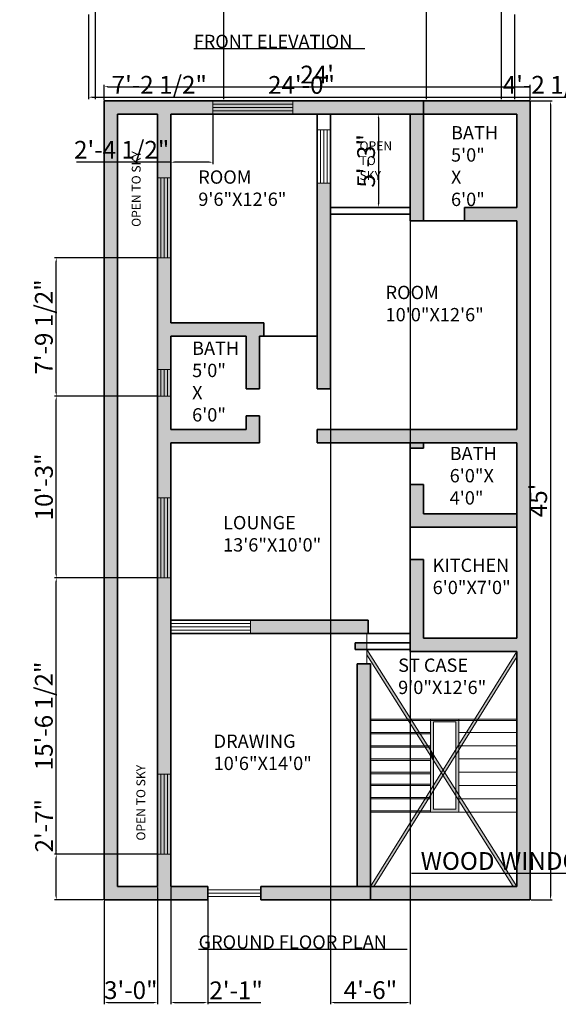
# Model space of a CAD drawing. Units: inches. Extents: x 2693 to 3501, y 1190 to 2292.
# Tile 1 of 4: x 2704 to 3068, y 1192 to 1858. Entities that reach past the tile are written whole.
import ezdxf

# ---------------------------------------------------------------- set-up
doc = ezdxf.new("R2010")
doc.units = ezdxf.units.IN
for name, color, linetype, lineweight in [('A-ANNO-DIMS', 2, 'Continuous', 18), ('A-ANNO-TEXT', 7, 'Continuous', 25), ('A-AREA-IDEN', 7, 'Continuous', 18), ('A-FLOR-STRS', 7, 'Continuous', 18), ('A-FLOR-STRS-PATT', 252, 'Continuous', 13), ('A-GLAZ', 4, 'Continuous', 18), ('A-WALL', 7, 'Continuous', 35), ('A-WALL-PATT', 252, 'Continuous', 13)]:
    doc.layers.add(name, color=color, linetype=linetype, lineweight=lineweight)
doc.styles.get("Standard").update_dxf_attribs({"font": 'arial.ttf'})
doc.dimstyles.new('ISO-25', dxfattribs={"dimtxt": 12, "dimasz": 2.5, "dimexe": 1.25, "dimexo": 0.625, "dimtad": 1, "dimdec": 1, "dimlunit": 3, "dimtxsty": 'Standard', "dimcen": 2.5, "dimadec": 0, "dimazin": 0, "dimtfac": 1, "dimtdec": 1, "dimtmove": 0, "dimatfit": 3, "dimfxl": 1, "dimarcsym": 0})

# ---------------------------------------------------------------- blocks, each defined once
blk = doc.blocks.new('Window - Wood Frame 36 in. Wide plan')
for p, q in [((0, 6), (0, 0)), ((0, 4.5), (36, 4.5)), ((36, 6), (36, 0)), ((0, 3), (36, 3)), ((0, 1.5), (36, 1.5))]:
    blk.add_line(p, q)
blk = doc.blocks.new('*D3')
at = {"layer": 'A-ANNO-DIMS', "color": 0, "lineweight": -2, "transparency": 16777216}
for p, q in [((2761.25, 1803.64), (2761.25, 1813.89)), ((2763.75, 1812.64), (3046.75, 1812.64)), ((3049.25, 1803.64), (3049.25, 1813.89))]:
    blk.add_line(p, q, dxfattribs=at)
at = {"layer": 'A-ANNO-DIMS', "color": 0, "transparency": 16777216}
for points in [[(2763.75, 1813.05), (2763.75, 1812.22), (2761.25, 1812.64)], [(3046.75, 1813.05), (3046.75, 1812.22), (3049.25, 1812.64)]]:
    blk.add_solid(points, dxfattribs=at)
at = {"layer": 'Defpoints', "color": 0, "transparency": 16777216}
for p in [(3049.25, 1812.64), (2761.25, 1803.02), (3049.25, 1803.02)]:
    blk.add_point(p, dxfattribs=at)
at = {"layer": 'A-ANNO-DIMS', "color": 0, "transparency": 16777216, "insert": (2905.25, 1819.29), "char_height": 12, "attachment_point": 5}
blk.add_mtext("24'", dxfattribs=at)
blk = doc.blocks.new('*D4')
at = {"layer": 'A-ANNO-DIMS', "color": 0, "lineweight": -2, "transparency": 16777216}
for p, q in [((3049.88, 1803.02), (3064.23, 1803.02)), ((3062.98, 1800.52), (3062.98, 1265.52)), ((3049.88, 1263.02), (3064.23, 1263.02))]:
    blk.add_line(p, q, dxfattribs=at)
at = {"layer": 'A-ANNO-DIMS', "color": 0, "transparency": 16777216}
for points in [[(3062.57, 1800.52), (3063.4, 1800.52), (3062.98, 1803.02)], [(3062.57, 1265.52), (3063.4, 1265.52), (3062.98, 1263.02)]]:
    blk.add_solid(points, dxfattribs=at)
at = {"layer": 'Defpoints', "color": 0, "transparency": 16777216}
for p in [(3049.25, 1803.02), (3049.25, 1263.02), (3062.98, 1263.02)]:
    blk.add_point(p, dxfattribs=at)
at = {"layer": 'A-ANNO-DIMS', "color": 0, "transparency": 16777216, "insert": (3056.26, 1533.02), "char_height": 12, "attachment_point": 5, "rotation": 90}
blk.add_mtext("45'", dxfattribs=at)
blk = doc.blocks.new('*D11')
at = {"layer": 'A-ANNO-DIMS', "color": 0, "lineweight": -2, "transparency": 16777216}
for p, q in [((3183.29, 1280.93), (2969.02, 1280.93)), ((3183.29, 1276.16), (3183.29, 1282.18)), ((3216.79, 1280.93), (3185.79, 1280.93)), ((3219.29, 1276.16), (3219.29, 1282.18))]:
    blk.add_line(p, q, dxfattribs=at)
at = {"layer": 'A-ANNO-DIMS', "color": 0, "transparency": 16777216}
for points in [[(3185.79, 1281.35), (3185.79, 1280.52), (3183.29, 1280.93)], [(3216.79, 1281.35), (3216.79, 1280.52), (3219.29, 1280.93)]]:
    blk.add_solid(points, dxfattribs=at)
at = {"layer": 'Defpoints', "color": 0, "transparency": 16777216}
for p in [(3183.29, 1280.93), (3183.29, 1275.53), (3219.29, 1275.53)]:
    blk.add_point(p, dxfattribs=at)
at = {"layer": 'A-ANNO-DIMS', "color": 0, "transparency": 16777216, "insert": (3074.91, 1287.77), "char_height": 12, "attachment_point": 5}
blk.add_mtext('WOOD WINDOW 3\'-0" TYP.', dxfattribs=at)
blk = doc.blocks.new('*D21')
at = {"layer": 'A-ANNO-DIMS', "color": 0, "lineweight": -2, "transparency": 16777216}
for p, q in [((2797.25, 1271.39), (2797.25, 1192.46)), ((2761.25, 1262.39), (2761.25, 1192.46)), ((2763.75, 1193.71), (2794.75, 1193.71))]:
    blk.add_line(p, q, dxfattribs=at)
at = {"layer": 'A-ANNO-DIMS', "color": 0, "transparency": 16777216}
for points in [[(2763.75, 1194.13), (2763.75, 1193.3), (2761.25, 1193.71)], [(2794.75, 1194.13), (2794.75, 1193.3), (2797.25, 1193.71)]]:
    blk.add_solid(points, dxfattribs=at)
at = {"layer": 'Defpoints', "color": 0, "transparency": 16777216}
for p in [(2797.25, 1272.02), (2761.25, 1263.02), (2797.25, 1193.71)]:
    blk.add_point(p, dxfattribs=at)
at = {"layer": 'A-ANNO-DIMS', "color": 0, "transparency": 16777216, "insert": (2779.25, 1200.47), "char_height": 12, "attachment_point": 5}
blk.add_mtext('3\'-0"', dxfattribs=at)
blk = doc.blocks.new('*D22')
at = {"layer": 'A-ANNO-DIMS', "color": 0, "lineweight": -2, "transparency": 16777216}
for p, q in [((2728.85, 1293.99), (2728.85, 1329.84)), ((2796.63, 1293.99), (2727.6, 1293.99)), ((2728.85, 1265.52), (2728.85, 1291.49)), ((2760.63, 1263.02), (2727.6, 1263.02))]:
    blk.add_line(p, q, dxfattribs=at)
at = {"layer": 'A-ANNO-DIMS', "color": 0, "transparency": 16777216}
for points in [[(2728.44, 1291.49), (2729.27, 1291.49), (2728.85, 1293.99)], [(2728.44, 1265.52), (2729.27, 1265.52), (2728.85, 1263.02)]]:
    blk.add_solid(points, dxfattribs=at)
at = {"layer": 'Defpoints', "color": 0, "transparency": 16777216}
for p in [(2728.85, 1293.99), (2797.25, 1293.99), (2761.25, 1263.02)]:
    blk.add_point(p, dxfattribs=at)
at = {"layer": 'A-ANNO-DIMS', "color": 0, "transparency": 16777216, "insert": (2722.2, 1313.17), "char_height": 12, "attachment_point": 5, "rotation": 90}
blk.add_mtext('2\'-7"', dxfattribs=at)
blk = doc.blocks.new('*D23')
at = {"layer": 'A-ANNO-DIMS', "color": 0, "lineweight": -2, "transparency": 16777216}
for p, q in [((2796.63, 1480.71), (2727.6, 1480.71)), ((2728.85, 1296.49), (2728.85, 1478.21)), ((2796.63, 1293.99), (2727.6, 1293.99))]:
    blk.add_line(p, q, dxfattribs=at)
at = {"layer": 'A-ANNO-DIMS', "color": 0, "transparency": 16777216}
for points in [[(2728.44, 1478.21), (2729.27, 1478.21), (2728.85, 1480.71)], [(2728.44, 1296.49), (2729.27, 1296.49), (2728.85, 1293.99)]]:
    blk.add_solid(points, dxfattribs=at)
at = {"layer": 'Defpoints', "color": 0, "transparency": 16777216}
for p in [(2728.85, 1480.71), (2797.25, 1480.71), (2797.25, 1293.99)]:
    blk.add_point(p, dxfattribs=at)
at = {"layer": 'A-ANNO-DIMS', "color": 0, "transparency": 16777216, "insert": (2722.02, 1387.35), "char_height": 12, "attachment_point": 5, "rotation": 90}
blk.add_mtext('15\'-6 1/2"', dxfattribs=at)
blk = doc.blocks.new('*D24')
at = {"layer": 'A-ANNO-DIMS', "color": 0, "lineweight": -2, "transparency": 16777216}
for p, q in [((2796.63, 1603.53), (2727.6, 1603.53)), ((2728.85, 1483.21), (2728.85, 1601.03)), ((2796.63, 1480.71), (2727.6, 1480.71))]:
    blk.add_line(p, q, dxfattribs=at)
at = {"layer": 'A-ANNO-DIMS', "color": 0, "transparency": 16777216}
for points in [[(2728.44, 1601.03), (2729.27, 1601.03), (2728.85, 1603.53)], [(2728.44, 1483.21), (2729.27, 1483.21), (2728.85, 1480.71)]]:
    blk.add_solid(points, dxfattribs=at)
at = {"layer": 'Defpoints', "color": 0, "transparency": 16777216}
for p in [(2728.85, 1603.53), (2797.25, 1603.53), (2797.25, 1480.71)]:
    blk.add_point(p, dxfattribs=at)
at = {"layer": 'A-ANNO-DIMS', "color": 0, "transparency": 16777216, "insert": (2722.1, 1542.12), "char_height": 12, "attachment_point": 5, "rotation": 90}
blk.add_mtext('10\'-3"', dxfattribs=at)
blk = doc.blocks.new('*D25')
at = {"layer": 'A-ANNO-DIMS', "color": 0, "lineweight": -2, "transparency": 16777216}
for p, q in [((2796.63, 1696.98), (2727.6, 1696.98)), ((2728.85, 1606.03), (2728.85, 1694.48)), ((2796.63, 1603.53), (2727.6, 1603.53))]:
    blk.add_line(p, q, dxfattribs=at)
at = {"layer": 'A-ANNO-DIMS', "color": 0, "transparency": 16777216}
for points in [[(2728.44, 1694.48), (2729.27, 1694.48), (2728.85, 1696.98)], [(2728.44, 1606.03), (2729.27, 1606.03), (2728.85, 1603.53)]]:
    blk.add_solid(points, dxfattribs=at)
at = {"layer": 'Defpoints', "color": 0, "transparency": 16777216}
for p in [(2728.85, 1696.98), (2797.25, 1696.98), (2797.25, 1603.53)]:
    blk.add_point(p, dxfattribs=at)
at = {"layer": 'A-ANNO-DIMS', "color": 0, "transparency": 16777216, "insert": (2722.02, 1650.25), "char_height": 12, "attachment_point": 5, "rotation": 90}
blk.add_mtext('7\'-9 1/2"', dxfattribs=at)
blk = doc.blocks.new('*D26')
at = {"layer": 'A-ANNO-DIMS', "color": 0, "lineweight": -2, "transparency": 16777216}
for p, q in [((2806.25, 1271.39), (2806.25, 1192.46)), ((2831.27, 1271.39), (2831.27, 1192.46)), ((2808.75, 1193.71), (2828.77, 1193.71)), ((2831.27, 1193.71), (2867.12, 1193.71))]:
    blk.add_line(p, q, dxfattribs=at)
at = {"layer": 'A-ANNO-DIMS', "color": 0, "transparency": 16777216}
for points in [[(2808.75, 1194.13), (2808.75, 1193.3), (2806.25, 1193.71)], [(2828.77, 1194.13), (2828.77, 1193.3), (2831.27, 1193.71)]]:
    blk.add_solid(points, dxfattribs=at)
at = {"layer": 'Defpoints', "color": 0, "transparency": 16777216}
for p in [(2806.25, 1272.02), (2831.27, 1272.02), (2831.27, 1193.71)]:
    blk.add_point(p, dxfattribs=at)
at = {"layer": 'A-ANNO-DIMS', "color": 0, "transparency": 16777216, "insert": (2850.45, 1200.36), "char_height": 12, "attachment_point": 5}
blk.add_mtext('2\'-1"', dxfattribs=at)
blk = doc.blocks.new('*D27')
at = {"layer": 'A-ANNO-DIMS', "color": 0, "lineweight": -2, "transparency": 16777216}
for p, q in [((2806.25, 1793.39), (2806.25, 1760.37)), ((2834.73, 1793.39), (2834.73, 1760.37)), ((2806.25, 1761.62), (2742.44, 1761.62)), ((2832.23, 1761.62), (2808.75, 1761.62))]:
    blk.add_line(p, q, dxfattribs=at)
at = {"layer": 'A-ANNO-DIMS', "color": 0, "transparency": 16777216}
for points in [[(2808.75, 1762.03), (2808.75, 1761.2), (2806.25, 1761.62)], [(2832.23, 1762.03), (2832.23, 1761.2), (2834.73, 1761.62)]]:
    blk.add_solid(points, dxfattribs=at)
at = {"layer": 'Defpoints', "color": 0, "transparency": 16777216}
for p in [(2806.25, 1794.02), (2834.73, 1794.02), (2806.25, 1761.62)]:
    blk.add_point(p, dxfattribs=at)
at = {"layer": 'A-ANNO-DIMS', "color": 0, "transparency": 16777216, "insert": (2773.1, 1768.45), "char_height": 12, "attachment_point": 5}
blk.add_mtext('2\'-4 1/2"', dxfattribs=at)
blk = doc.blocks.new('*D28')
at = {"layer": 'A-ANNO-DIMS', "color": 0, "lineweight": -2, "transparency": 16777216}
for p, q in [((2914.25, 1730.39), (2914.25, 1192.46)), ((2968.25, 1730.39), (2968.25, 1192.46)), ((2916.75, 1193.71), (2965.75, 1193.71))]:
    blk.add_line(p, q, dxfattribs=at)
at = {"layer": 'A-ANNO-DIMS', "color": 0, "transparency": 16777216}
for points in [[(2916.75, 1194.13), (2916.75, 1193.3), (2914.25, 1193.71)], [(2965.75, 1194.13), (2965.75, 1193.3), (2968.25, 1193.71)]]:
    blk.add_solid(points, dxfattribs=at)
at = {"layer": 'Defpoints', "color": 0, "transparency": 16777216}
for p in [(2914.25, 1731.02), (2968.25, 1731.02), (2968.25, 1193.71)]:
    blk.add_point(p, dxfattribs=at)
at = {"layer": 'A-ANNO-DIMS', "color": 0, "transparency": 16777216, "insert": (2941.25, 1200.47), "char_height": 12, "attachment_point": 5}
blk.add_mtext('4\'-6"', dxfattribs=at)
blk = doc.blocks.new('*D29')
at = {"layer": 'A-ANNO-DIMS', "color": 0, "lineweight": -2, "transparency": 16777216}
for p, q in [((2914.88, 1794.02), (2947.9, 1794.02)), ((2946.65, 1791.52), (2946.65, 1733.52)), ((2914.88, 1731.02), (2947.9, 1731.02))]:
    blk.add_line(p, q, dxfattribs=at)
at = {"layer": 'A-ANNO-DIMS', "color": 0, "transparency": 16777216}
for points in [[(2946.24, 1791.52), (2947.07, 1791.52), (2946.65, 1794.02)], [(2946.24, 1733.52), (2947.07, 1733.52), (2946.65, 1731.02)]]:
    blk.add_solid(points, dxfattribs=at)
at = {"layer": 'Defpoints', "color": 0, "transparency": 16777216}
for p in [(2914.25, 1794.02), (2914.25, 1731.02), (2946.65, 1731.02)]:
    blk.add_point(p, dxfattribs=at)
at = {"layer": 'A-ANNO-DIMS', "color": 0, "transparency": 16777216, "insert": (2939.9, 1762.52), "char_height": 12, "attachment_point": 5, "rotation": 90}
blk.add_mtext('5\'-3"', dxfattribs=at)
blk = doc.blocks.new('*D36')
at = {"layer": 'A-ANNO-DIMS', "color": 0, "lineweight": -2, "transparency": 16777216}
for p, q in [((2841.85, 1945.66), (2841.85, 1804.29)), ((2755.18, 1889.87), (2755.18, 1804.29)), ((2757.68, 1805.54), (2839.35, 1805.54))]:
    blk.add_line(p, q, dxfattribs=at)
at = {"layer": 'A-ANNO-DIMS', "color": 0, "transparency": 16777216}
for points in [[(2757.68, 1805.95), (2757.68, 1805.12), (2755.18, 1805.54)], [(2839.35, 1805.95), (2839.35, 1805.12), (2841.85, 1805.54)]]:
    blk.add_solid(points, dxfattribs=at)
at = {"layer": 'Defpoints', "color": 0, "transparency": 16777216}
for p in [(2841.85, 1946.28), (2755.18, 1890.49), (2841.85, 1805.54)]:
    blk.add_point(p, dxfattribs=at)
at = {"layer": 'A-ANNO-DIMS', "color": 0, "transparency": 16777216, "insert": (2798.51, 1812.37), "char_height": 12, "attachment_point": 5}
blk.add_mtext('7\'-2 1/2"', dxfattribs=at)
blk = doc.blocks.new('*D41')
at = {"layer": 'A-ANNO-DIMS', "color": 0, "lineweight": -2, "transparency": 16777216}
for p, q in [((2978.99, 1889.87), (2978.99, 1804.29)), ((3029.68, 1889.87), (3029.68, 1804.29)), ((2981.49, 1805.54), (3027.18, 1805.54)), ((3029.68, 1805.54), (3093.77, 1805.54))]:
    blk.add_line(p, q, dxfattribs=at)
at = {"layer": 'A-ANNO-DIMS', "color": 0, "transparency": 16777216}
for points in [[(2981.49, 1805.95), (2981.49, 1805.12), (2978.99, 1805.54)], [(3027.18, 1805.95), (3027.18, 1805.12), (3029.68, 1805.54)]]:
    blk.add_solid(points, dxfattribs=at)
at = {"layer": 'Defpoints', "color": 0, "transparency": 16777216}
for p in [(2978.99, 1890.49), (3029.68, 1890.49), (3029.68, 1805.54)]:
    blk.add_point(p, dxfattribs=at)
at = {"layer": 'A-ANNO-DIMS', "color": 0, "transparency": 16777216, "insert": (3062.97, 1812.37), "char_height": 12, "attachment_point": 5}
blk.add_mtext('4\'-2 1/2"', dxfattribs=at)
blk = doc.blocks.new('*D46')
at = {"layer": 'A-ANNO-DIMS', "color": 0, "lineweight": -2, "transparency": 16777216}
for p, q in [((2750.68, 1861.37), (2750.68, 1804.29)), ((3038.68, 1861.37), (3038.68, 1804.29)), ((2753.18, 1805.54), (3036.18, 1805.54))]:
    blk.add_line(p, q, dxfattribs=at)
at = {"layer": 'A-ANNO-DIMS', "color": 0, "transparency": 16777216}
for points in [[(2753.18, 1805.95), (2753.18, 1805.12), (2750.68, 1805.54)], [(3036.18, 1805.95), (3036.18, 1805.12), (3038.68, 1805.54)]]:
    blk.add_solid(points, dxfattribs=at)
at = {"layer": 'Defpoints', "color": 0, "transparency": 16777216}
for p in [(2750.68, 1861.99), (3038.68, 1861.99), (3038.68, 1805.54)]:
    blk.add_point(p, dxfattribs=at)
at = {"layer": 'A-ANNO-DIMS', "color": 0, "transparency": 16777216, "insert": (2894.68, 1812.29), "char_height": 12, "attachment_point": 5}
blk.add_mtext('24\'-0"', dxfattribs=at)

msp = doc.modelspace()

# ---------------------------------------------------------------- hatches: boundary and pattern name
at = {"layer": 'A-FLOR-STRS-PATT'}
h = msp.add_hatch(color=256, dxfattribs=at)
h.dxf.hatch_style = 1
h.paths.add_polyline_path([(2969.2, 1384.27), (2966.83, 1384.27), (2971.89, 1376.27), (2974.26, 1376.27)])
h.paths.add_polyline_path([(2938.79, 1432.3), (2938.79, 1428.56), (2966.2, 1385.27), (2968.56, 1385.27)])
h.paths.add_polyline_path([(2968.56, 1385.27), (2966.2, 1385.27), (2966.83, 1384.27), (2969.2, 1384.27)])
h.paths.add_polyline_path([(2981.95, 1385.27), (2968.56, 1385.27), (2969.2, 1384.27), (2981.95, 1384.27)])
h.paths.add_polyline_path([(2966.2, 1385.27), (2941.25, 1385.27), (2941.25, 1384.27), (2966.83, 1384.27)])
h.paths.add_polyline_path([(2971.89, 1376.27), (2941.25, 1376.27), (2941.25, 1375.27), (2972.53, 1375.27)])
h.paths.add_polyline_path([(2981.95, 1376.27), (2974.26, 1376.27), (2974.89, 1375.27), (2981.95, 1375.27)])
h.paths.add_polyline_path([(2974.26, 1376.27), (2971.89, 1376.27), (2972.53, 1375.27), (2974.89, 1375.27)])
h.paths.add_polyline_path([(2974.89, 1375.27), (2972.53, 1375.27), (2977.59, 1367.27), (2979.96, 1367.27)])
h.paths.add_polyline_path([(2979.96, 1367.27), (2977.59, 1367.27), (2978.22, 1366.27), (2980.59, 1366.27)])
h.paths.add_polyline_path([(2981.95, 1367.27), (2979.96, 1367.27), (2980.59, 1366.27), (2981.95, 1366.27)])
h.paths.add_polyline_path([(2977.59, 1367.27), (2941.25, 1367.27), (2941.25, 1366.27), (2978.22, 1366.27)])
h.paths.add_polyline_path([(2980.59, 1366.27), (2978.22, 1366.27), (2981.95, 1360.38), (2981.95, 1364.12)])
h.paths.add_polyline_path([(2981.95, 1358.27), (2941.25, 1358.27), (2941.25, 1357.27), (2981.95, 1357.27)])
h.paths.add_polyline_path([(2981.95, 1349.27), (2941.25, 1349.27), (2941.25, 1348.27), (2981.95, 1348.27)])
h.paths.add_polyline_path([(2981.95, 1364.12), (2981.95, 1360.38), (2983.95, 1357.22), (2983.95, 1360.96)], flags=17)
h.paths.add_polyline_path([(2983.95, 1360.96), (2983.95, 1357.22), (2989.17, 1348.97), (2990.35, 1350.86)], flags=17)
h.paths.add_polyline_path([(2990.35, 1350.86), (2989.17, 1348.97), (2990.36, 1347.1), (2991.53, 1348.98)], flags=17)
h.paths.add_polyline_path([(2999.01, 1360.99), (2999.01, 1364.77), (2990.35, 1350.86), (2991.53, 1348.98)], flags=17)
h.paths.add_polyline_path([(2974.9, 1322.27), (2972.54, 1322.27), (2941.25, 1272.02), (2943.61, 1272.02)])
h.paths.add_polyline_path([(3008.44, 1322.27), (3006.08, 1322.27), (3037.89, 1272.02), (3040.25, 1272.02)])
h.paths.add_polyline_path([(2981.95, 1323.27), (2975.52, 1323.27), (2974.9, 1322.27), (2981.95, 1322.27)])
h.paths.add_polyline_path([(2975.52, 1323.27), (2973.17, 1323.27), (2972.54, 1322.27), (2974.9, 1322.27)])
h.paths.add_polyline_path([(2973.17, 1323.27), (2941.25, 1323.27), (2941.25, 1322.27), (2972.54, 1322.27)])
h.paths.add_polyline_path([(2978.77, 1332.27), (2941.25, 1332.27), (2941.25, 1331.27), (2978.15, 1331.27)])
h.paths.add_polyline_path([(2981.95, 1341.27), (2941.25, 1341.27), (2941.25, 1340.27), (2981.95, 1340.27)])
h.paths.add_polyline_path([(2981.13, 1332.27), (2978.77, 1332.27), (2978.15, 1331.27), (2980.5, 1331.27)])
h.paths.add_polyline_path([(2981.95, 1333.59), (2981.95, 1337.37), (2978.77, 1332.27), (2981.13, 1332.27)])
h.paths.add_polyline_path([(2980.5, 1331.27), (2978.15, 1331.27), (2973.17, 1323.27), (2975.52, 1323.27)])
h.paths.add_polyline_path([(2983.95, 1336.8), (2981.95, 1333.59), (2981.95, 1322.27), (3001.01, 1322.27), (3001.01, 1330.28), (2999.01, 1333.44), (2999.01, 1324.27), (2983.95, 1324.27)])
h.paths.add_polyline_path([(2981.95, 1332.27), (2981.13, 1332.27), (2980.5, 1331.27), (2981.95, 1331.27)])
h.paths.add_polyline_path([(2983.95, 1336.8), (2983.95, 1340.59), (2981.95, 1337.37), (2981.95, 1333.59)])
h.paths.add_polyline_path([(2983.95, 1383.27), (2999.01, 1383.27), (2999.01, 1364.77), (3001.01, 1367.98), (3001.01, 1385.27), (2981.95, 1385.27), (2981.95, 1337.37), (2983.95, 1340.59)])
h.paths.add_polyline_path([(3001.01, 1367.98), (2999.01, 1364.77), (2999.01, 1360.99), (3001.01, 1364.2)], flags=17)
h.paths.add_polyline_path([(3001.01, 1364.2), (2999.01, 1360.99), (2999.01, 1337.18), (3001.01, 1334.02)])
h.paths.add_polyline_path([(2991.53, 1348.98), (2990.36, 1347.1), (2999.01, 1333.44), (2999.01, 1337.18)])
h.paths.add_polyline_path([(2990.36, 1347.1), (2989.17, 1348.97), (2983.95, 1340.59), (2983.95, 1336.8)])
h.paths.add_polyline_path([(3002.75, 1331.27), (3001.01, 1331.27), (3001.01, 1330.28), (3006.08, 1322.27), (3008.44, 1322.27)])
h.paths.add_polyline_path([(3001.01, 1334.02), (2999.01, 1337.18), (2999.01, 1333.44), (3001.01, 1330.28)])
h.paths.add_polyline_path([(3001.01, 1334.02), (3001.01, 1331.27), (3002.75, 1331.27)])
h.paths.add_polyline_path([(3040.25, 1427.23), (3040.25, 1431.02), (3011.77, 1385.27), (3014.13, 1385.27)])
h.paths.add_polyline_path([(3013.5, 1384.27), (3011.15, 1384.27), (3006.17, 1376.27), (3008.52, 1376.27)])
h.paths.add_polyline_path([(3014.13, 1385.27), (3011.77, 1385.27), (3011.15, 1384.27), (3013.5, 1384.27)])
h.paths.add_polyline_path([(3008.52, 1376.27), (3006.17, 1376.27), (3001.01, 1367.98), (3001.01, 1367.27), (3002.92, 1367.27)])
h.paths.add_polyline_path([(3002.92, 1367.27), (3001.01, 1367.27), (3001.01, 1364.2)])
h = msp.add_hatch(color=256, dxfattribs=at)
h.dxf.hatch_style = 1
h.paths.add_polyline_path([(2983.95, 1360.96), (2981.95, 1364.12), (2981.95, 1360.38), (2983.95, 1357.22)])
at = {"layer": 'A-WALL-PATT'}
h = msp.add_hatch(color=256, dxfattribs=at)
h.dxf.hatch_style = 1
h.paths.add_polyline_path([(2806.25, 1572.02), (2866.25, 1572.02), (2866.25, 1590.19), (2857.25, 1590.19), (2857.25, 1581.02), (2806.25, 1581.02), (2806.25, 1644.02), (2857.25, 1644.02), (2857.25, 1608.49), (2866.25, 1608.49), (2866.25, 1644.02), (2869.25, 1644.02), (2869.25, 1653.02), (2806.25, 1653.02), (2806.25, 1794.02), (3040.25, 1794.02), (3040.25, 1731.02), (3004.91, 1731.02), (3004.91, 1722.02), (3040.25, 1722.02), (3040.25, 1581.02), (2905.25, 1581.02), (2905.25, 1572.02), (3040.25, 1572.02), (3040.25, 1440.02), (2977.25, 1440.02), (2977.25, 1493.16), (2968.25, 1493.16), (2968.25, 1431.02), (3040.25, 1431.02), (3040.25, 1272.02), (2941.25, 1272.02), (2941.25, 1263.02), (3049.25, 1263.02), (3049.25, 1803.02), (2761.25, 1803.02), (2761.25, 1263.02), (2831.27, 1263.02), (2831.27, 1272.02), (2806.25, 1272.02)])
h.paths.add_polyline_path([(2770.25, 1794.02), (2797.25, 1794.02), (2797.25, 1272.02), (2770.25, 1272.02)], flags=16)
h.paths.add_polyline_path([(2806.25, 1480.71), (2797.25, 1480.71), (2797.25, 1347.99), (2806.25, 1347.99)], flags=17)
h.paths.add_polyline_path([(2939.65, 1452.02), (2860.25, 1452.02), (2860.25, 1443.02), (2939.65, 1443.02)], flags=17)
h.paths.add_polyline_path([(2941.25, 1272.02), (2867.27, 1272.02), (2867.27, 1263.02), (2941.25, 1263.02)], flags=17)
h.paths.add_polyline_path([(2914.25, 1722.02), (2914.25, 1747.49), (2905.25, 1747.49), (2905.25, 1644.02), (2905.25, 1608.49), (2914.25, 1608.49)], flags=17)
h.paths.add_polyline_path([(2977.25, 1794.02), (2968.25, 1794.02), (2968.25, 1722.02), (2977.25, 1722.02)], flags=17)
h.paths.add_polyline_path([(2792.46, 1301.22), (2792.46, 1361.05), (2780.09, 1361.05), (2780.09, 1301.22)], flags=8)
h.paths.add_polyline_path([(2789.3, 1716.02), (2789.3, 1775.84), (2776.94, 1775.84), (2776.94, 1716.02)], flags=8)
h = msp.add_hatch(color=256, dxfattribs=at)
h.dxf.hatch_style = 1
h.paths.add_polyline_path([(2977.25, 1572.02), (2968.25, 1572.02), (2968.25, 1568.42), (2977.25, 1568.42)])
h.paths.add_polyline_path([(2977.25, 1543.76), (2968.25, 1543.76), (2968.25, 1515.02), (3040.25, 1515.02), (3040.25, 1524.02), (2977.25, 1524.02)])
h = msp.add_hatch(color=256, dxfattribs=at)
h.dxf.hatch_style = 1
h.paths.add_polyline_path([(2806.25, 1480.71), (2797.25, 1480.71), (2797.25, 1347.99), (2806.25, 1347.99)])
h = msp.add_hatch(color=256, dxfattribs=at)
h.dxf.hatch_style = 1
h.paths.add_polyline_path([(3293.27, 1426.01), (3284.27, 1426.01), (3284.27, 1275.53), (3293.27, 1275.53)])
h.paths.add_polyline_path([(3290.81, 1440.32), (3282.91, 1440.32), (3282.91, 1435.82), (3290.81, 1435.82)])
h.paths.add_polyline_path([(2941.25, 1422.49), (2932.25, 1422.49), (2932.25, 1272.02), (2941.25, 1272.02)])
h.paths.add_polyline_path([(2938.79, 1436.8), (2930.89, 1436.8), (2930.89, 1432.3), (2938.79, 1432.3)])

# ---------------------------------------------------------------- linework, layer by layer
at = {"layer": 'A-ANNO-TEXT'}
for p, q in [((2821.79, 1838.44), (2937.53, 1838.44)), ((2825.1, 1229.72), (2966.07, 1229.72))]:
    msp.add_line(p, q, dxfattribs=at)
at = {"layer": 'A-FLOR-STRS'}
for p, q in [((2938.79, 1443.02), (2938.79, 1422.49)), ((2938.79, 1432.3), (3040.25, 1272.02)), ((3040.25, 1431.02), (2941.25, 1272.02)), ((2938.79, 1428.56), (3037.89, 1272.02)), ((3040.25, 1427.23), (2943.61, 1272.02)), ((2941.25, 1385.27), (3040.25, 1385.27)), ((2941.25, 1384.27), (3040.25, 1384.27)), ((2941.25, 1376.27), (2981.95, 1376.27)), ((2941.25, 1375.27), (2981.95, 1375.27)), ((3001.01, 1376.27), (3040.25, 1376.27)), ((2941.25, 1367.27), (2981.95, 1367.27)), ((2941.25, 1366.27), (2981.95, 1366.27)), ((3001.01, 1367.27), (3040.25, 1367.27)), ((2941.25, 1358.27), (2981.95, 1358.27)), ((3001.01, 1358.27), (3040.25, 1358.27)), ((2941.25, 1357.27), (2981.95, 1357.27)), ((2941.25, 1349.27), (2981.95, 1349.27)), ((2941.25, 1348.27), (2981.95, 1348.27)), ((3001.01, 1349.27), (3040.25, 1349.27)), ((2941.25, 1341.27), (2981.95, 1341.27)), ((2941.25, 1340.27), (2981.95, 1340.27)), ((3001.01, 1340.27), (3040.25, 1340.27)), ((2941.25, 1331.27), (2941.25, 1332.27)), ((2941.25, 1332.27), (2981.95, 1332.27)), ((2941.25, 1331.27), (2981.95, 1331.27)), ((2981.95, 1332.27), (2981.95, 1331.27)), ((3001.01, 1331.27), (3040.25, 1331.27)), ((2941.25, 1322.27), (2941.25, 1323.27)), ((2941.25, 1323.27), (2981.95, 1323.27)), ((2941.25, 1322.27), (3040.25, 1322.27)), ((2981.95, 1323.27), (2981.95, 1322.27))]:
    msp.add_line(p, q, dxfattribs=at)
for points in [[(2981.95, 1385.27), (3001.01, 1385.27), (3001.01, 1322.27), (2981.95, 1322.27)], [(2983.95, 1383.27), (2999.01, 1383.27), (2999.01, 1324.27), (2983.95, 1324.27)]]:
    msp.add_lwpolyline(points, close=True, dxfattribs=at)
at = {"layer": 'A-WALL'}
for p, q in [((2761.25, 1803.02), (3049.25, 1803.02)), ((2761.25, 1263.02), (2761.25, 1803.02)), ((2977.25, 1794.02), (2977.25, 1803.02)), ((3049.25, 1803.02), (3049.25, 1263.02)), ((2770.25, 1794.02), (2797.25, 1794.02)), ((2770.25, 1272.02), (2770.25, 1794.02)), ((2797.25, 1272.02), (2797.25, 1794.02)), ((2806.25, 1794.02), (3040.25, 1794.02)), ((2806.25, 1653.02), (2806.25, 1794.02)), ((2905.25, 1644.02), (2905.25, 1794.02)), ((2914.25, 1722.02), (2914.25, 1794.02)), ((2968.25, 1722.02), (2968.25, 1794.02)), ((2977.25, 1722.02), (2977.25, 1794.02)), ((3040.25, 1794.02), (3040.25, 1731.02)), ((2914.25, 1731.02), (2968.25, 1731.02)), ((3004.91, 1731.02), (3040.25, 1731.02)), ((3004.91, 1731.02), (3004.91, 1722.02)), ((2914.25, 1726.52), (2968.25, 1726.52)), ((2914.25, 1608.49), (2914.25, 1722.02)), ((2968.25, 1722.02), (3040.25, 1722.02)), ((3040.25, 1722.02), (3040.25, 1581.02)), ((2806.25, 1653.02), (2869.25, 1653.02)), ((2869.25, 1644.02), (2869.25, 1653.02)), ((2806.25, 1644.02), (2857.25, 1644.02)), ((2806.25, 1581.02), (2806.25, 1644.02)), ((2857.25, 1608.49), (2857.25, 1644.02)), ((2866.25, 1644.02), (2905.25, 1644.02)), ((2866.25, 1608.49), (2866.25, 1644.02)), ((2866.25, 1644.02), (2869.25, 1644.02)), ((2905.25, 1608.49), (2905.25, 1644.02)), ((2857.25, 1608.49), (2866.25, 1608.49)), ((2905.25, 1608.49), (2914.25, 1608.49)), ((2857.25, 1581.02), (2857.25, 1590.19)), ((2866.25, 1590.19), (2857.25, 1590.19)), ((2866.25, 1572.02), (2866.25, 1590.19)), ((2806.25, 1581.02), (2857.25, 1581.02)), ((2905.25, 1581.02), (3040.25, 1581.02)), ((2905.25, 1572.02), (2905.25, 1581.02)), ((2806.25, 1572.02), (2866.25, 1572.02)), ((2806.25, 1272.02), (2806.25, 1572.02)), ((2905.25, 1572.02), (3040.25, 1572.02)), ((2968.25, 1572.02), (2968.25, 1568.42)), ((2977.25, 1572.02), (2977.25, 1568.42)), ((3040.25, 1572.02), (3040.25, 1440.02)), ((2968.25, 1568.42), (2977.25, 1568.42)), ((2968.25, 1543.76), (2968.25, 1568.42)), ((2968.25, 1543.76), (2968.25, 1431.02)), ((2968.25, 1543.76), (2977.25, 1543.76)), ((2977.25, 1543.76), (2977.25, 1524.02)), ((2977.25, 1524.02), (3040.25, 1524.02)), ((2968.25, 1515.02), (3040.25, 1515.02)), ((2968.25, 1493.16), (2977.25, 1493.16)), ((2977.25, 1493.16), (2977.25, 1440.02)), ((2806.25, 1452.02), (2939.65, 1452.02)), ((2939.65, 1452.02), (2939.65, 1443.02)), ((2806.25, 1443.02), (2968.25, 1443.02)), ((2977.25, 1440.02), (3040.25, 1440.02)), ((2941.25, 1436.8), (2930.89, 1436.8)), ((2932.13, 1436.8), (2930.89, 1436.8)), ((2930.89, 1436.8), (2930.89, 1432.3)), ((2930.89, 1432.3), (2941.25, 1432.3)), ((2968.11, 1436.8), (2941.25, 1436.8)), ((2968.11, 1432.3), (2941.25, 1432.3)), ((2968.25, 1431.02), (3040.25, 1431.02)), ((3040.25, 1431.02), (3040.25, 1272.02)), ((3040.25, 1272.02), (3040.25, 1431.02)), ((2932.25, 1422.49), (2932.25, 1272.02)), ((2932.25, 1422.49), (2941.25, 1422.49)), ((2941.25, 1422.49), (2941.25, 1263.02)), ((2797.25, 1272.02), (2770.25, 1272.02)), ((2831.27, 1272.02), (2806.25, 1272.02)), ((2831.27, 1272.02), (2831.27, 1263.02)), ((3040.25, 1272.02), (2867.27, 1272.02)), ((2867.27, 1263.02), (2867.27, 1272.02)), ((2831.27, 1263.02), (2761.25, 1263.02)), ((3049.25, 1263.02), (2867.27, 1263.02))]:
    msp.add_line(p, q, dxfattribs=at)

# ---------------------------------------------------------------- block references
at = {"layer": 'A-GLAZ', "xscale": 1.5, "yscale": 1.5}
for p in [(2834.73, 1794.02), (2806.25, 1443.02)]:
    msp.add_blockref('Window - Wood Frame 36 in. Wide plan', p, dxfattribs=at)
at = {"layer": 'A-GLAZ', "yscale": 1.5}
for p, rotation in [((2914.25, 1747.49), 90), ((2867.27, 1272.02), 180)]:
    msp.add_blockref('Window - Wood Frame 36 in. Wide plan', p, dxfattribs=dict(at, rotation=rotation))
at = {"layer": 'A-GLAZ', "yscale": 1.5, "rotation": 90}
for p, xscale in [((2806.25, 1696.98), 1.5), ((2806.25, 1603.53), 0.5), ((2806.25, 1480.71), 1.5), ((2806.25, 1293.99), 1.5)]:
    msp.add_blockref('Window - Wood Frame 36 in. Wide plan', p, dxfattribs=dict(at, xscale=xscale))

# ---------------------------------------------------------------- texts
at = {"layer": 'A-ANNO-TEXT', "char_height": 9, "attachment_point": 1}
for s, insert in [('FRONT ELEVATION', (2821.79, 1847.75)), ('GROUND FLOOR PLAN', (2825.1, 1239.03))]:
    msp.add_mtext_dynamic_manual_height_columns(s, width=140.9736, gutter_width=12.5, heights=[0], dxfattribs=dict(at, insert=insert))
at = {"layer": 'A-AREA-IDEN', "char_height": 9, "attachment_point": 1}
for s, width, insert in [('BATH\\P5\'0"\\PX\\P6\'0"', 1.6077, (2995.75, 1786)), ('ROOM\\P9\'6"X12\'6"', 1.6077, (2824.89, 1756.08)), ('ROOM\\P10\'0"X12\'6"', 1.6077, (2951.52, 1678.08)), ('BATH\\P5\'0"\\PX\\P6\'0"', 1.6077, (2820.71, 1640.38)), ('BATH\\P6\'0"X\\P4\'0"', 1.6077, (2994.86, 1569.24)), ('LOUNGE 13\'6"X10\'0"', 77.2555, (2841.63, 1522.49)), ('KITCHEN\\P6\'0"X7\'0"', 1.6077, (2983.34, 1493.7)), ('ST CASE\\P9\'0"X12\'6"', 77.2555, (2960.01, 1426.16)), ('DRAWING 10\'6"X14\'0"', 77.2555, (2835.26, 1374.8))]:
    msp.add_mtext_dynamic_manual_height_columns(s, width=width, gutter_width=12.5, heights=[0], dxfattribs=dict(at, insert=insert))
at = {"layer": 'A-AREA-IDEN', "insert": (2933.92, 1775.69), "char_height": 6, "attachment_point": 1}
msp.add_mtext('OPEN \\PTO \\PSKY', dxfattribs=at)
at = {"layer": 'A-AREA-IDEN', "char_height": 6, "attachment_point": 1, "rotation": 90}
for insert in [(2779.92, 1717.92), (2783.07, 1303.13)]:
    msp.add_mtext_dynamic_manual_height_columns('OPEN TO SKY', width=75.3875, gutter_width=12.5, heights=[0], dxfattribs=dict(at, insert=insert))

# ---------------------------------------------------------------- dimensions: what is measured, and where the dimension line sits
at = {"layer": 'A-ANNO-DIMS'}
for base, p1, p2, override, picture, middle in [((2841.85, 1805.54), (2755.18, 1890.49), (2841.85, 1946.28), {"dimdec": 1, "dimlfac": 1, "dimrnd": 0, "dimzin": 1, "dimdsep": 46, "dimlunit": 4, "dimfrac": 2}, '*D36', (2798.51, 1812.37)), ((3029.68, 1805.54), (2978.99, 1890.49), (3029.68, 1890.49), {"dimdec": 1, "dimlfac": 1, "dimrnd": 0, "dimzin": 1, "dimdsep": 46, "dimlunit": 4, "dimfrac": 2}, '*D41', (3062.97, 1812.37)), ((3038.68, 1805.54), (2750.68, 1861.99), (3038.68, 1861.99), {"dimdec": 1, "dimlfac": 1, "dimrnd": 0, "dimzin": 1, "dimdsep": 46, "dimlunit": 4, "dimfrac": 2}, '*D46', (2894.68, 1812.29)), ((3049.25, 1812.64), (2761.25, 1803.02), (3049.25, 1803.02), {"dimclrd": 0, "dimclre": 0, "dimclrt": 0}, '*D3', (2905.25, 1819.29)), ((2968.25, 1193.71), (2914.25, 1731.02), (2968.25, 1731.02), {"dimdec": 1, "dimlfac": 1, "dimrnd": 0, "dimzin": 1, "dimdsep": 46, "dimlunit": 4, "dimfrac": 2}, '*D28', (2941.25, 1200.47)), ((2797.25, 1193.71), (2761.25, 1263.02), (2797.25, 1272.02), {"dimdec": 1, "dimlfac": 1, "dimrnd": 0, "dimzin": 1, "dimdsep": 46, "dimlunit": 4, "dimfrac": 2}, '*D21', (2779.25, 1200.47)), ((2831.27, 1193.71), (2806.25, 1272.02), (2831.27, 1272.02), {"dimdec": 1, "dimlfac": 1, "dimrnd": 0, "dimzin": 1, "dimdsep": 46, "dimlunit": 4, "dimfrac": 2}, '*D26', (2850.45, 1200.36))]:
    dim = msp.add_linear_dim(base=base, p1=p1, p2=p2, dimstyle='ISO-25', override=override, dxfattribs=at)
    dim.commit()
    dim.dimension.update_dxf_attribs({"geometry": picture, "text_midpoint": middle})
for base, p1, p2, angle, override, picture, middle in [((3062.98, 1263.02), (3049.25, 1803.02), (3049.25, 1263.02), 90, {"dimclrd": 0, "dimclre": 0, "dimclrt": 0}, '*D4', (3056.26, 1533.02)), ((2806.25, 1761.62), (2834.73, 1794.02), (2806.25, 1794.02), 180, {"dimdec": 1, "dimlfac": 1, "dimrnd": 0, "dimzin": 1, "dimdsep": 46, "dimlunit": 4, "dimfrac": 2}, '*D27', (2773.1, 1768.45)), ((2946.65, 1731.02), (2914.25, 1794.02), (2914.25, 1731.02), 270, {"dimdec": 1, "dimlfac": 1, "dimrnd": 0, "dimzin": 1, "dimdsep": 46, "dimlunit": 4, "dimfrac": 2}, '*D29', (2939.9, 1762.52)), ((2728.854, 1696.9833), (2797.254, 1603.5262), (2797.254, 1696.9833), 90, {"dimdec": 1, "dimlfac": 1, "dimrnd": 0, "dimzin": 1, "dimdsep": 46, "dimlunit": 4, "dimfrac": 2}, '*D25', (2722.0243, 1650.2548)), ((2728.85, 1603.53), (2797.25, 1480.71), (2797.25, 1603.53), 90, {"dimdec": 1, "dimlfac": 1, "dimrnd": 0, "dimzin": 1, "dimdsep": 46, "dimlunit": 4, "dimfrac": 2}, '*D24', (2722.1, 1542.12)), ((2728.85, 1480.71), (2797.25, 1293.99), (2797.25, 1480.71), 90, {"dimdec": 1, "dimlfac": 1, "dimrnd": 0, "dimzin": 1, "dimdsep": 46, "dimlunit": 4, "dimfrac": 2}, '*D23', (2722.02, 1387.35)), ((2728.85, 1293.99), (2761.25, 1263.02), (2797.25, 1293.99), 90, {"dimdec": 1, "dimlfac": 1, "dimrnd": 0, "dimzin": 1, "dimdsep": 46, "dimlunit": 4, "dimfrac": 2}, '*D22', (2722.2, 1313.17))]:
    dim = msp.add_linear_dim(base=base, p1=p1, p2=p2, angle=angle, dimstyle='ISO-25', override=override, dxfattribs=at)
    dim.commit()
    dim.dimension.update_dxf_attribs({"geometry": picture, "text_midpoint": middle})
dim = msp.add_linear_dim(base=(3183.29, 1280.93), p1=(3219.29, 1275.53), p2=(3183.29, 1275.53), angle=180, text='WOOD WINDOW <> TYP.', dimstyle='ISO-25', override={"dimdec": 1, "dimlfac": 1, "dimrnd": 0, "dimzin": 1, "dimdsep": 46, "dimlunit": 4, "dimfrac": 2}, dxfattribs=at)
dim.commit()
dim.dimension.update_dxf_attribs({"geometry": '*D11', "text_midpoint": (3074.91, 1287.77)})

doc.saveas('drawing.dxf')
